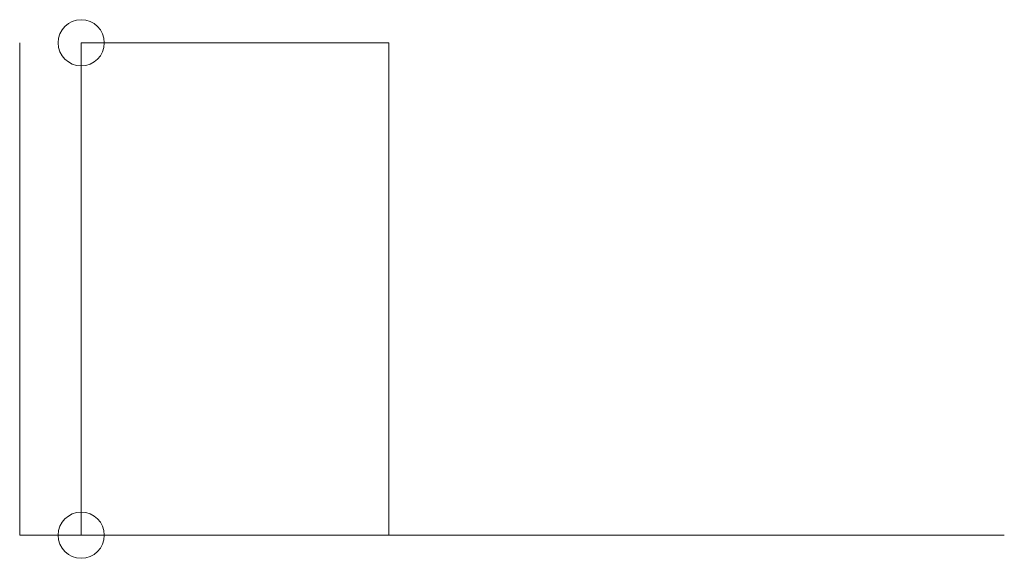
# Model space of a CAD drawing. Units: millimetres. Extents: x 457 to 585, y -3 to 67.
import ezdxf

# ---------------------------------------------------------------- set-up
doc = ezdxf.new("R2010")
doc.units = ezdxf.units.MM
doc.layers.add('M-CONS', color=8, linetype='Continuous', lineweight=13)

msp = doc.modelspace()

# ---------------------------------------------------------------- linework, layer by layer
at = {"layer": 'M-CONS'}
msp.add_line((504.57, 64, 88.22), (492.57, 64, 88.22), dxfattribs=at)
at = {"layer": 'M-CONS', "extrusion": (0, -1, 0)}
for p, q in [((504.57, 0, 80.22), (456.57, 0, 80.22)), ((456.57, 0, 80.22), (456.57, 0, 120.22)), ((504.57, 0, 80.22), (504.57, 0, 64.22)), ((536.57, 0, 64.22), (536.57, 0, 80.22)), ((536.57, 0, 80.22), (564.57, 0, 80.22))]:
    msp.add_line(p, q, dxfattribs=at)
at = {"layer": 'M-CONS', "extrusion": (-1, 0, 0), "elevation": -456.57}
msp.add_lwpolyline([(0, 80.22), (-64, 80.22), (-64, 120.22), (0, 120.22)], close=True, dxfattribs=at)
at = {"layer": 'M-CONS', "elevation": 80.22}
msp.add_lwpolyline([(504.57, 64), (504.57, 0), (464.57, 0), (464.57, 64)], close=True, dxfattribs=at)
at = {"layer": 'M-CONS', "extrusion": (-1, 0, 0), "elevation": -456.57}
msp.add_lwpolyline([(-48, 96.22), (-48, 80.22), (-16, 80.22), (-16, 96.22, 1)], format="xyb", close=True, dxfattribs=at)
at = {"layer": 'M-CONS'}
for centre in [(464.57, 64, 120.22), (464.57, 0, 120.22)]:
    msp.add_circle(centre, 3, dxfattribs=at)
at = {"layer": 'M-CONS', "extrusion": (-1, 0, 0)}
msp.add_circle((-32, 96.22, -456.57), 3, dxfattribs=at)
at = {"layer": 'M-CONS', "extrusion": (0, -1, 0)}
for centre, radius in [((520.57, 64.22), 8), ((564.57, 100.22), 12.5)]:
    msp.add_circle(centre, radius, dxfattribs=at)
for centre, radius, start, end in [((520.57, 64.22), 16, 180, 0), ((564.57, 100.22), 20, 270, 90)]:
    msp.add_arc(centre, radius, start, end, dxfattribs=at)

doc.saveas('drawing.dxf')
